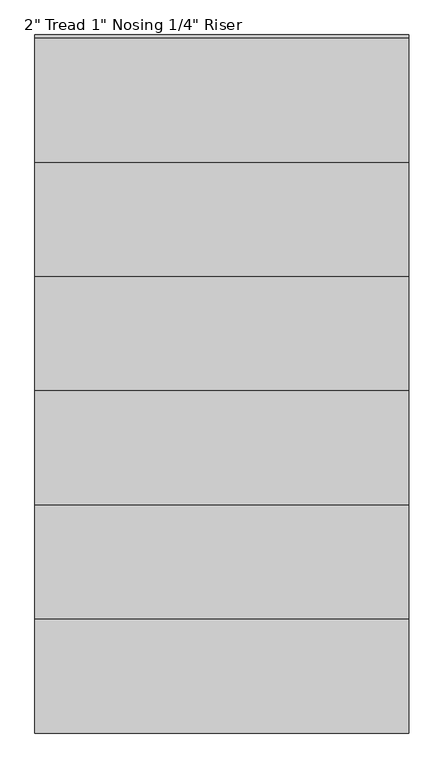
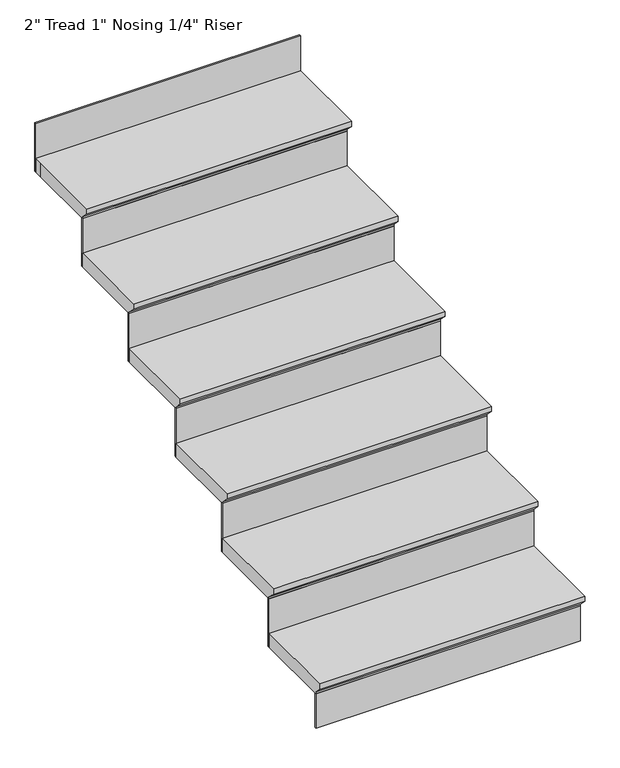
"""IFC4 building model written with IfcOpenShell, lengths in millimetres: stair flight geometry."""

from ifc_helpers import new_model, si_unit, origin, place, context, project, spatial, faceted_brep, source, transform, mapped, element, save


def stair_flight_bb85c52a(model_context):
    return source(origin(), model_context, "Body", "Brep", [
        faceted_brep([(-12594.3954771, 1037.2129676, 3359.15), (-12594.3954771, 1037.2129676, 3378.2), (-13508.7954771, 1037.2129676, 3378.2), (-13508.7954771, 1037.2129676, 3359.15), (-12594.3954771, 1062.6129676, 3333.75), (-13508.7954771, 1062.6129676, 3333.75), (-12594.3954771, 1342.0129676, 3378.2), (-13508.7954771, 1342.0129676, 3378.2), (-13508.7954771, 1062.6129676, 3327.4), (-13508.7954771, 1342.0129676, 3327.4), (-12594.3954771, 1342.0129676, 3327.4), (-12594.3954771, 1062.6129676, 3327.4)], [[[0, 1, 2, 3]], [[4, 0, 3, 5]], [[2, 1, 6, 7]], [[8, 9, 10, 11]], [[2, 7, 9, 8, 5, 3]], [[8, 11, 4, 5]], [[6, 1, 0, 4, 11, 10]], [[7, 6, 10, 9]]]),
        faceted_brep([(-12594.3954771, 1062.6129676, 3327.4), (-12594.3954771, 1062.6129676, 3200.4), (-12594.3954771, 1068.9629676, 3200.4), (-12594.3954771, 1068.9629676, 3327.4), (-13508.7954771, 1062.6129676, 3327.4), (-13508.7954771, 1068.9629676, 3327.4), (-13508.7954771, 1068.9629676, 3200.4), (-13508.7954771, 1062.6129676, 3200.4)], [[[0, 1, 2, 3]], [[4, 5, 6, 7]], [[1, 0, 4, 7]], [[2, 1, 7, 6]], [[3, 2, 6, 5]], [[0, 3, 5, 4]]]),
        faceted_brep([(-12594.3954771, 1342.0129676, 3505.2), (-12594.3954771, 1342.0129676, 3327.4), (-12594.3954771, 1348.3629676, 3327.4), (-12594.3954771, 1348.3629676, 3505.2), (-13508.7954771, 1342.0129676, 3505.2), (-13508.7954771, 1348.3629676, 3505.2), (-13508.7954771, 1348.3629676, 3327.4), (-13508.7954771, 1342.0129676, 3327.4)], [[[0, 1, 2, 3]], [[4, 5, 6, 7]], [[1, 0, 4, 7]], [[2, 1, 7, 6]], [[3, 2, 6, 5]], [[0, 3, 5, 4]]]),
        faceted_brep([(-13508.7954771, 1316.6129676, 3556.0), (-12594.3954771, 1316.6129676, 3556.0), (-12594.3954771, 1621.4129676, 3556.0), (-13508.7954771, 1621.4129676, 3556.0), (-13508.7954771, 1342.0129676, 3505.2), (-13508.7954771, 1621.4129676, 3505.2), (-12594.3954771, 1621.4129676, 3505.2), (-12594.3954771, 1342.0129676, 3505.2), (-13508.7954771, 1342.0129676, 3511.55), (-13508.7954771, 1316.6129676, 3536.95), (-12594.3954771, 1342.0129676, 3511.55), (-12594.3954771, 1316.6129676, 3536.95)], [[[0, 1, 2, 3]], [[4, 5, 6, 7]], [[0, 3, 5, 4, 8, 9]], [[4, 7, 10, 8]], [[2, 1, 11, 10, 7, 6]], [[3, 2, 6, 5]], [[11, 1, 0, 9]], [[10, 11, 9, 8]]]),
        faceted_brep([(-12594.3954771, 1621.4129676, 3683.0), (-12594.3954771, 1621.4129676, 3505.2), (-12594.3954771, 1627.7629676, 3505.2), (-12594.3954771, 1627.7629676, 3683.0), (-13508.7954771, 1621.4129676, 3683.0), (-13508.7954771, 1627.7629676, 3683.0), (-13508.7954771, 1627.7629676, 3505.2), (-13508.7954771, 1621.4129676, 3505.2)], [[[0, 1, 2, 3]], [[4, 5, 6, 7]], [[1, 0, 4, 7]], [[2, 1, 7, 6]], [[3, 2, 6, 5]], [[0, 3, 5, 4]]]),
        faceted_brep([(-13508.7954771, 1596.0129676, 3733.8), (-12594.3954771, 1596.0129676, 3733.8), (-12594.3954771, 1900.8129676, 3733.8), (-13508.7954771, 1900.8129676, 3733.8), (-13508.7954771, 1621.4129676, 3683.0), (-13508.7954771, 1900.8129676, 3683.0), (-12594.3954771, 1900.8129676, 3683.0), (-12594.3954771, 1621.4129676, 3683.0), (-13508.7954771, 1621.4129676, 3689.35), (-13508.7954771, 1596.0129676, 3714.75), (-12594.3954771, 1621.4129676, 3689.35), (-12594.3954771, 1596.0129676, 3714.75)], [[[0, 1, 2, 3]], [[4, 5, 6, 7]], [[0, 3, 5, 4, 8, 9]], [[4, 7, 10, 8]], [[2, 1, 11, 10, 7, 6]], [[3, 2, 6, 5]], [[11, 1, 0, 9]], [[10, 11, 9, 8]]]),
        faceted_brep([(-12594.3954771, 1900.8129676, 3860.8), (-12594.3954771, 1900.8129676, 3683.0), (-12594.3954771, 1907.1629676, 3683.0), (-12594.3954771, 1907.1629676, 3860.8), (-13508.7954771, 1900.8129676, 3860.8), (-13508.7954771, 1907.1629676, 3860.8), (-13508.7954771, 1907.1629676, 3683.0), (-13508.7954771, 1900.8129676, 3683.0)], [[[0, 1, 2, 3]], [[4, 5, 6, 7]], [[1, 0, 4, 7]], [[2, 1, 7, 6]], [[3, 2, 6, 5]], [[0, 3, 5, 4]]]),
        faceted_brep([(-13508.7954771, 1875.4129676, 3911.6), (-12594.3954771, 1875.4129676, 3911.6), (-12594.3954771, 2180.2129676, 3911.6), (-13508.7954771, 2180.2129676, 3911.6), (-13508.7954771, 1900.8129676, 3860.8), (-13508.7954771, 2180.2129676, 3860.8), (-12594.3954771, 2180.2129676, 3860.8), (-12594.3954771, 1900.8129676, 3860.8), (-13508.7954771, 1900.8129676, 3867.15), (-13508.7954771, 1875.4129676, 3892.55), (-12594.3954771, 1900.8129676, 3867.15), (-12594.3954771, 1875.4129676, 3892.55)], [[[0, 1, 2, 3]], [[4, 5, 6, 7]], [[0, 3, 5, 4, 8, 9]], [[4, 7, 10, 8]], [[2, 1, 11, 10, 7, 6]], [[3, 2, 6, 5]], [[11, 1, 0, 9]], [[10, 11, 9, 8]]]),
        faceted_brep([(-12594.3954771, 2180.2129676, 4038.6), (-12594.3954771, 2180.2129676, 3860.8), (-12594.3954771, 2186.5629676, 3860.8), (-12594.3954771, 2186.5629676, 4038.6), (-13508.7954771, 2180.2129676, 4038.6), (-13508.7954771, 2186.5629676, 4038.6), (-13508.7954771, 2186.5629676, 3860.8), (-13508.7954771, 2180.2129676, 3860.8)], [[[0, 1, 2, 3]], [[4, 5, 6, 7]], [[1, 0, 4, 7]], [[2, 1, 7, 6]], [[3, 2, 6, 5]], [[0, 3, 5, 4]]]),
        faceted_brep([(-13508.7954771, 2154.8129676, 4089.4), (-12594.3954771, 2154.8129676, 4089.4), (-12594.3954771, 2459.6129676, 4089.4), (-13508.7954771, 2459.6129676, 4089.4), (-13508.7954771, 2180.2129676, 4038.6), (-13508.7954771, 2459.6129676, 4038.6), (-12594.3954771, 2459.6129676, 4038.6), (-12594.3954771, 2180.2129676, 4038.6), (-13508.7954771, 2180.2129676, 4044.95), (-13508.7954771, 2154.8129676, 4070.35), (-12594.3954771, 2180.2129676, 4044.95), (-12594.3954771, 2154.8129676, 4070.35)], [[[0, 1, 2, 3]], [[4, 5, 6, 7]], [[0, 3, 5, 4, 8, 9]], [[4, 7, 10, 8]], [[2, 1, 11, 10, 7, 6]], [[3, 2, 6, 5]], [[11, 1, 0, 9]], [[10, 11, 9, 8]]]),
        faceted_brep([(-12594.3954771, 2739.0129676, 4394.2), (-12594.3954771, 2739.0129676, 4216.4), (-12594.3954771, 2745.3629676, 4216.4), (-12594.3954771, 2745.3629676, 4394.2), (-13508.7954771, 2739.0129676, 4394.2), (-13508.7954771, 2745.3629676, 4394.2), (-13508.7954771, 2745.3629676, 4216.4), (-13508.7954771, 2739.0129676, 4216.4)], [[[0, 1, 2, 3]], [[4, 5, 6, 7]], [[1, 0, 4, 7]], [[2, 1, 7, 6]], [[3, 2, 6, 5]], [[0, 3, 5, 4]]]),
        faceted_brep([(-12594.3954771, 2459.6129676, 4216.4), (-12594.3954771, 2459.6129676, 4038.6), (-12594.3954771, 2465.9629676, 4038.6), (-12594.3954771, 2465.9629676, 4216.4), (-13508.7954771, 2459.6129676, 4216.4), (-13508.7954771, 2465.9629676, 4216.4), (-13508.7954771, 2465.9629676, 4038.6), (-13508.7954771, 2459.6129676, 4038.6)], [[[0, 1, 2, 3]], [[4, 5, 6, 7]], [[1, 0, 4, 7]], [[2, 1, 7, 6]], [[3, 2, 6, 5]], [[0, 3, 5, 4]]]),
        faceted_brep([(-13508.7954771, 2739.0129676, 4267.2), (-13508.7954771, 2713.6129676, 4267.2), (-13508.7954771, 2434.2129676, 4267.2), (-12594.3954771, 2434.2129676, 4267.2), (-12594.3954771, 2713.6129676, 4267.2), (-12594.3954771, 2739.0129676, 4267.2), (-13508.7954771, 2713.6129676, 4216.4), (-13508.7954771, 2739.0129676, 4216.4), (-12594.3954771, 2739.0129676, 4216.4), (-12594.3954771, 2713.6129676, 4216.4), (-12594.3954771, 2459.6129676, 4216.4), (-13508.7954771, 2459.6129676, 4216.4), (-13508.7954771, 2459.6129676, 4222.75), (-13508.7954771, 2434.2129676, 4248.15), (-12594.3954771, 2459.6129676, 4222.75), (-12594.3954771, 2434.2129676, 4248.15)], [[[0, 1, 2, 3, 4, 5]], [[6, 7, 8, 9, 10, 11]], [[1, 0, 7, 6]], [[2, 1, 6, 11, 12, 13]], [[11, 10, 14, 12]], [[4, 3, 15, 14, 10, 9]], [[5, 4, 9, 8]], [[0, 5, 8, 7]], [[15, 3, 2, 13]], [[14, 15, 13, 12]]]),
    ])


if __name__ == "__main__":
    model = new_model("IFC4")
    model_context = context("Model", 3, world=origin())
    ifc_project = project(units=[si_unit("LENGTHUNIT", "METRE", prefix="MILLI")], contexts=[model_context])
    site = spatial("IfcSite", under=ifc_project)
    building = spatial("IfcBuilding", under=site)
    placement = place(None, origin())
    stair_flight_shape = stair_flight_bb85c52a(model_context)
    element("IfcStairFlight", 1, ObjectType="2\" Tread 1\" Nosing 1/4\" Riser", at=placement, inside=building, context=model_context, shape_type="MappedRepresentation", body=[
        mapped(stair_flight_shape, transform((0.0, 0.0, 0.0), x_axis=(1.0, 0.0, 0.0), y_axis=(0.0, 1.0, 0.0), z_axis=(0.0, 0.0, 1.0))),
    ])
    save(model, "model.ifc")
